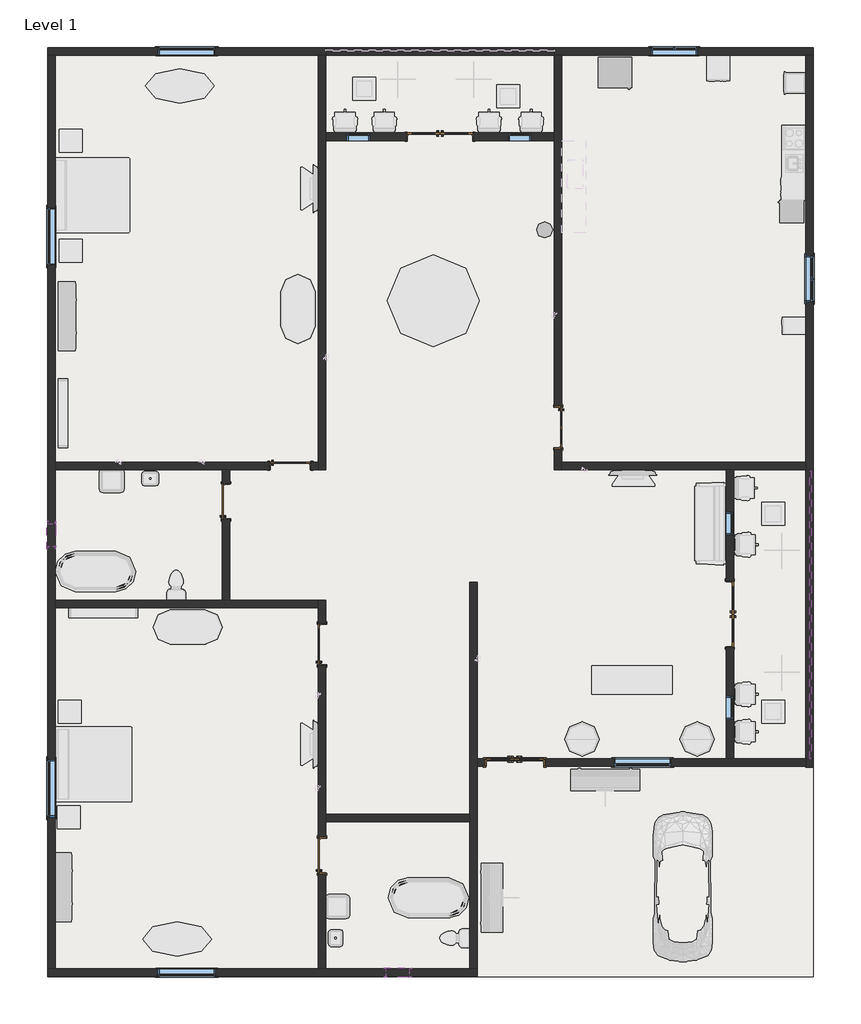
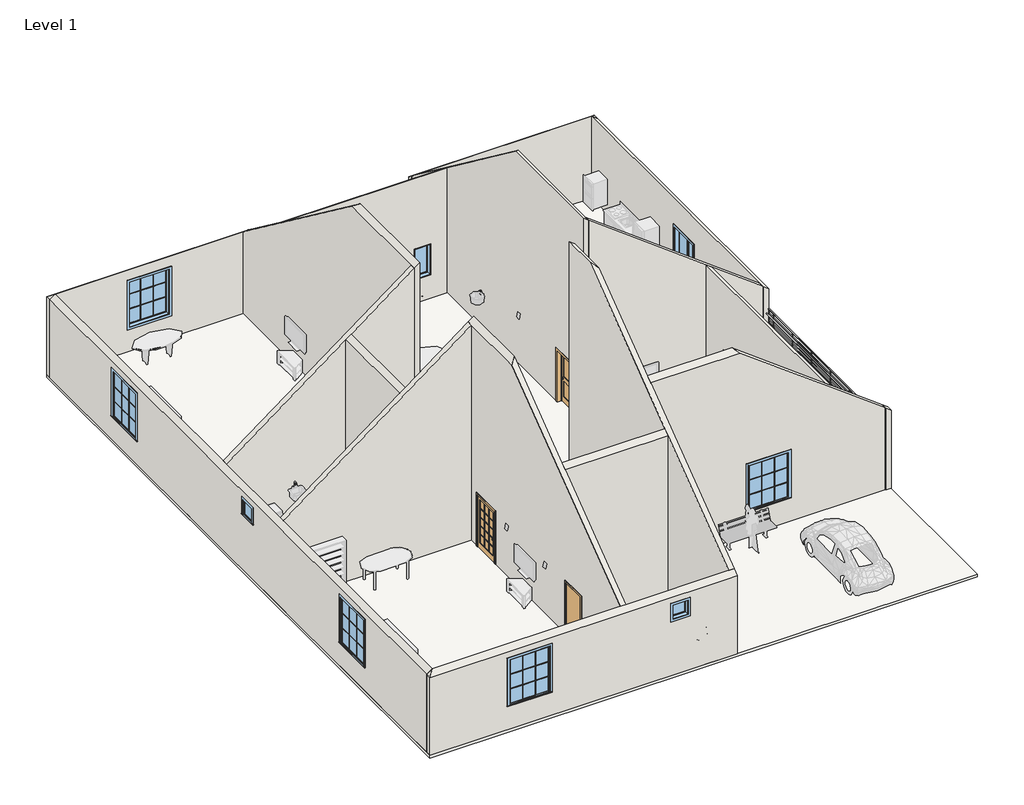
# One storey, part 1 of 2: 20 walls, 13 windows, 8 doors, 1 railing, 1 slab.
# Revit data of these elements (continued)
# Elements 27, 29 (IfcWall, "Generic - 8\"")
#   Top Offset = 0' - 0"
#   Base Offset = 0' - 0"
#   Unconnected Height = 4' - 0"
#   wall height = 4' - 0"
#   Phase Created = New Construction
#   Base Constraint = Level 1
#   Materials on its faces: "Brick, Common"
# Element 31 (IfcWindow, "Casement 3x3 with Trim : 60\" x 72\"")
#   Mark = "1"
#   Phase Created = New Construction
#   Materials on its faces: "Sash", "Glass", "Trim"
# Element 32 (IfcWindow, "Casement 3x3 with Trim : 60\" x 72\"")
#   Mark = "2"
#   Phase Created = New Construction
#   Materials on its faces: "Sash", "Glass", "Trim"
# Element 33 (IfcWindow, "Casement 3x3 with Trim : 60\" x 72\"")
#   Mark = "3"
#   Phase Created = New Construction
#   Materials on its faces: "Sash", "Glass", "Trim"
# Element 34 (IfcWindow, "Casement 3x3 with Trim : 60\" x 72\"")
#   Mark = "4"
#   Phase Created = New Construction
#   Materials on its faces: "Sash", "Glass", "Trim"
# Element 35 (IfcWindow, "Casement 3x3 with Trim : 60\" x 72\"")
#   Mark = "5"
#   Phase Created = New Construction
#   Materials on its faces: "Sash", "Glass", "Trim"
# Element 36 (IfcWindow, "Casement Dbl with Trim : 48\" x 48\"")
#   Mark = "13"
#   Phase Created = New Construction
#   Materials on its faces: "Sash", "Trim", "Glass"
# Element 37 (IfcWindow, "Casement Dbl with Trim : 48\" x 48\"")
#   Mark = "14"
#   Phase Created = New Construction
#   Materials on its faces: "Sash", "Trim", "Glass"
# Element 38 (IfcWindow, "Fixed : 24\" x 48\"")
#   Mark = "9"
#   Phase Created = New Construction
#   Materials on its faces: "Sash", "Glass"
# Element 39 (IfcWindow, "Fixed : 24\" x 48\"")
#   Mark = "10"
#   Phase Created = New Construction
#   Materials on its faces: "Sash", "Glass"
# Element 40 (IfcWindow, "Fixed : 24\" x 48\"")
#   Mark = "11"
#   Phase Created = New Construction
#   Materials on its faces: "Sash", "Glass"
# Element 41 (IfcWindow, "Fixed : 24\" x 48\"")
#   Mark = "12"
#   Phase Created = New Construction
#   Materials on its faces: "Sash", "Glass"
# Element 42 (IfcWindow, "Transom with Trim : 24\" x 24\"")
#   Mark = "6"
#   Phase Created = New Construction
#   Materials on its faces: "Sash", "Trim", "Glass"
# Element 43 (IfcWindow, "Transom with Trim : 24\" x 24\"")
#   Mark = "7"
#   Phase Created = New Construction
#   Materials on its faces: "Sash", "Trim", "Glass"
# Materials
#   "Cherry": class "Wood", colour RGB 226 177 128, transparency 0, Description = "Prunus Serotina", Cost = 0
#   "Glass": class "Glass", colour RGB 0 128 192, transparency 0.75, Description = "Soda Lime Glass", Cost = 0
#   "Aluminum": class "Metal", colour RGB 247 247 247, transparency 0, Description = "Aluminum 6061", Cost = 0
#   "Concrete, Lightweight": class "Concrete", colour RGB 142 141 140, transparency 0, Description = "Lightweight concrete", Cost = 0
#   "Metal Deck": class "Metal", colour RGB 199 199 199, transparency 0, Description = "Steel, mill finish", Cost = 0
#   "Brick, Common": class "Masonry", colour RGB 170 98 104, transparency 0, Description = "Common brick", Cost = 0
#   "Sash": class "Wood", colour RGB 224 178 126, transparency 0
#   "Trim": class "Wood", colour RGB 224 178 126, transparency 0
# Room at (-11268.389, 6197.334) mm, phase "New Construction", upper level "Level 1", upper offset 10' - 0", lower offset 0' - 0"
#   Number = "1"
#   Name = "BED ROOM"
# Room at (2195.235, 6197.334) mm, phase "New Construction", upper level "Level 1", upper offset 10' - 0", lower offset 0' - 0"
#   Number = "2"
#   Name = "KITCHEN"
# Room at (-4467.116, 4935.179) mm, phase "New Construction", upper level "Level 1", upper offset 10' - 0", lower offset 0' - 0"
#   Number = "3"
# Room at (0, -3898.809) mm, phase "New Construction", upper level "Level 1", upper offset 10' - 0", lower offset 0' - 0"
#   Number = "4"
#   Name = "LIVING AREA"
# Room at (-12383.374, -1900.74) mm, phase "New Construction", upper level "Level 1", upper offset 10' - 0", lower offset 0' - 0"
#   Number = "5"
#   Name = "TOILET"
# Room at (-11412.091, -8144.703) mm, phase "New Construction", upper level "Level 1", upper offset 10' - 0", lower offset 0' - 0"
#   Number = "6"
#   Name = "BED ROOM"
# Room at (-5362.385, -11474.816) mm, phase "New Construction", upper level "Level 1", upper offset 10' - 0", lower offset 0' - 0"
#   Number = "7"
#   Name = "TOILET"
# Room at (0, -10808.794) mm, phase "New Construction", upper level "Level 1", upper offset 10' - 0", lower offset 0' - 0"
#   Number = "8"
# Room at (4794.461, -3982.061) mm, phase "New Construction", upper level "Level 1", upper offset 10' - 0", lower offset 0' - 0"
#   Number = "9"
#   Name = "BALCONY"
# Room at (-4467.116, 9556.237) mm, phase "New Construction", upper level "Level 1", upper offset 10' - 0", lower offset 0' - 0"
#   Number = "10"
#   Name = "BALCONY"
